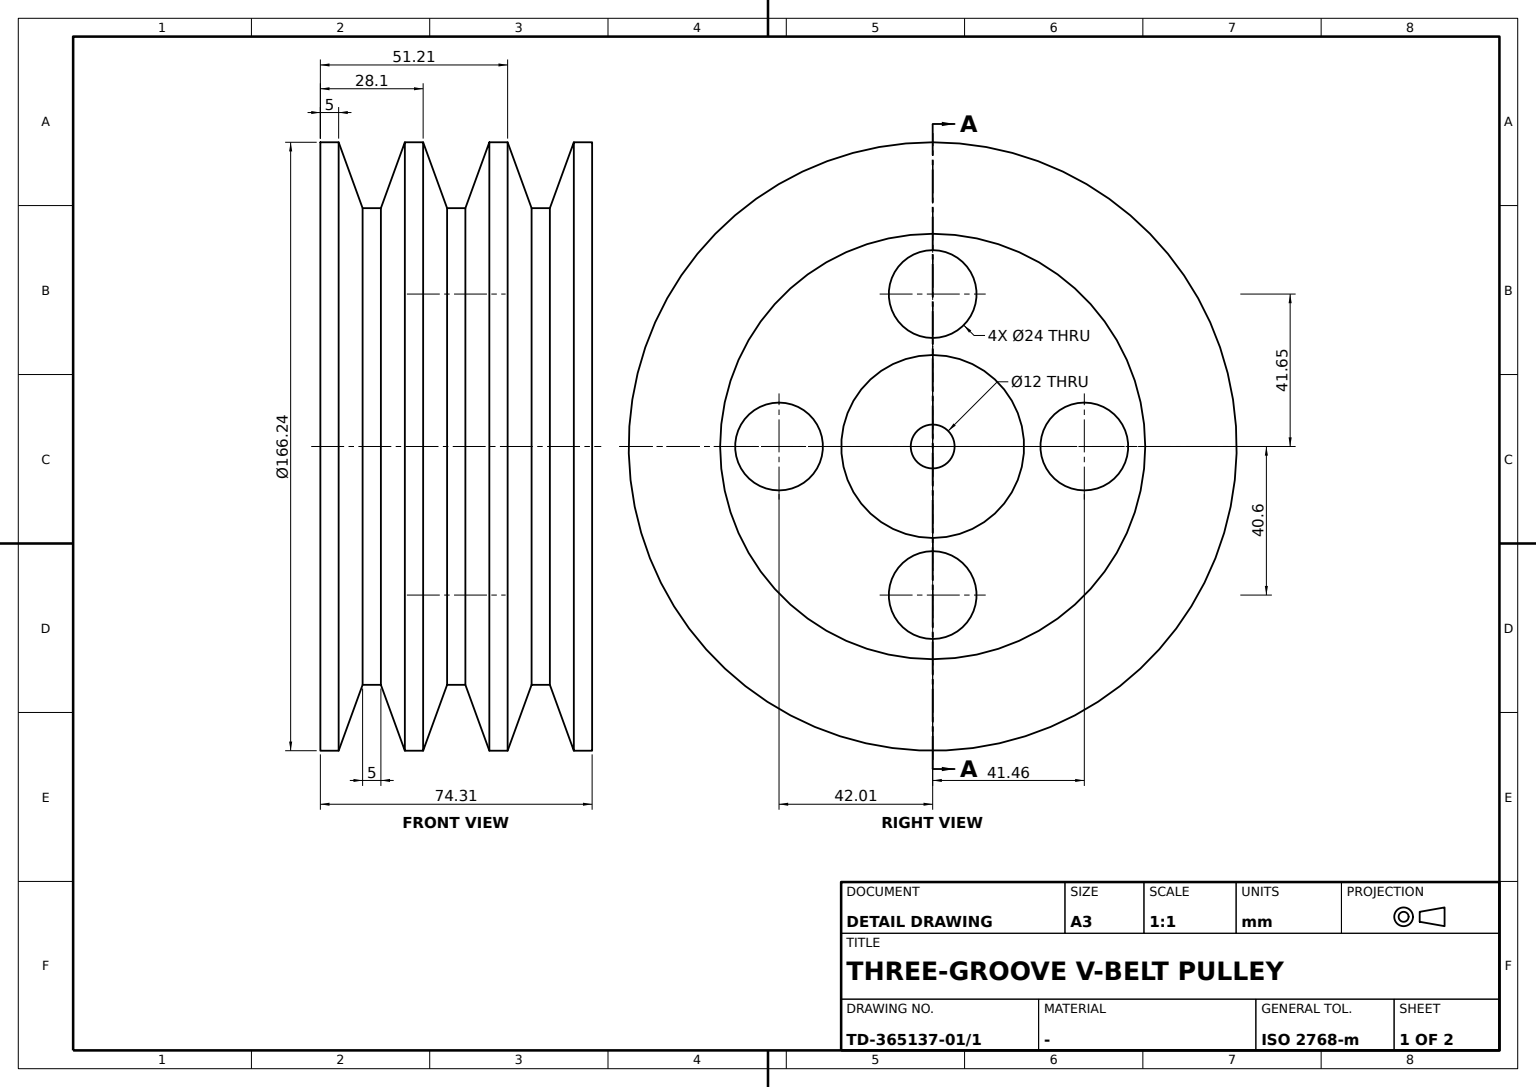
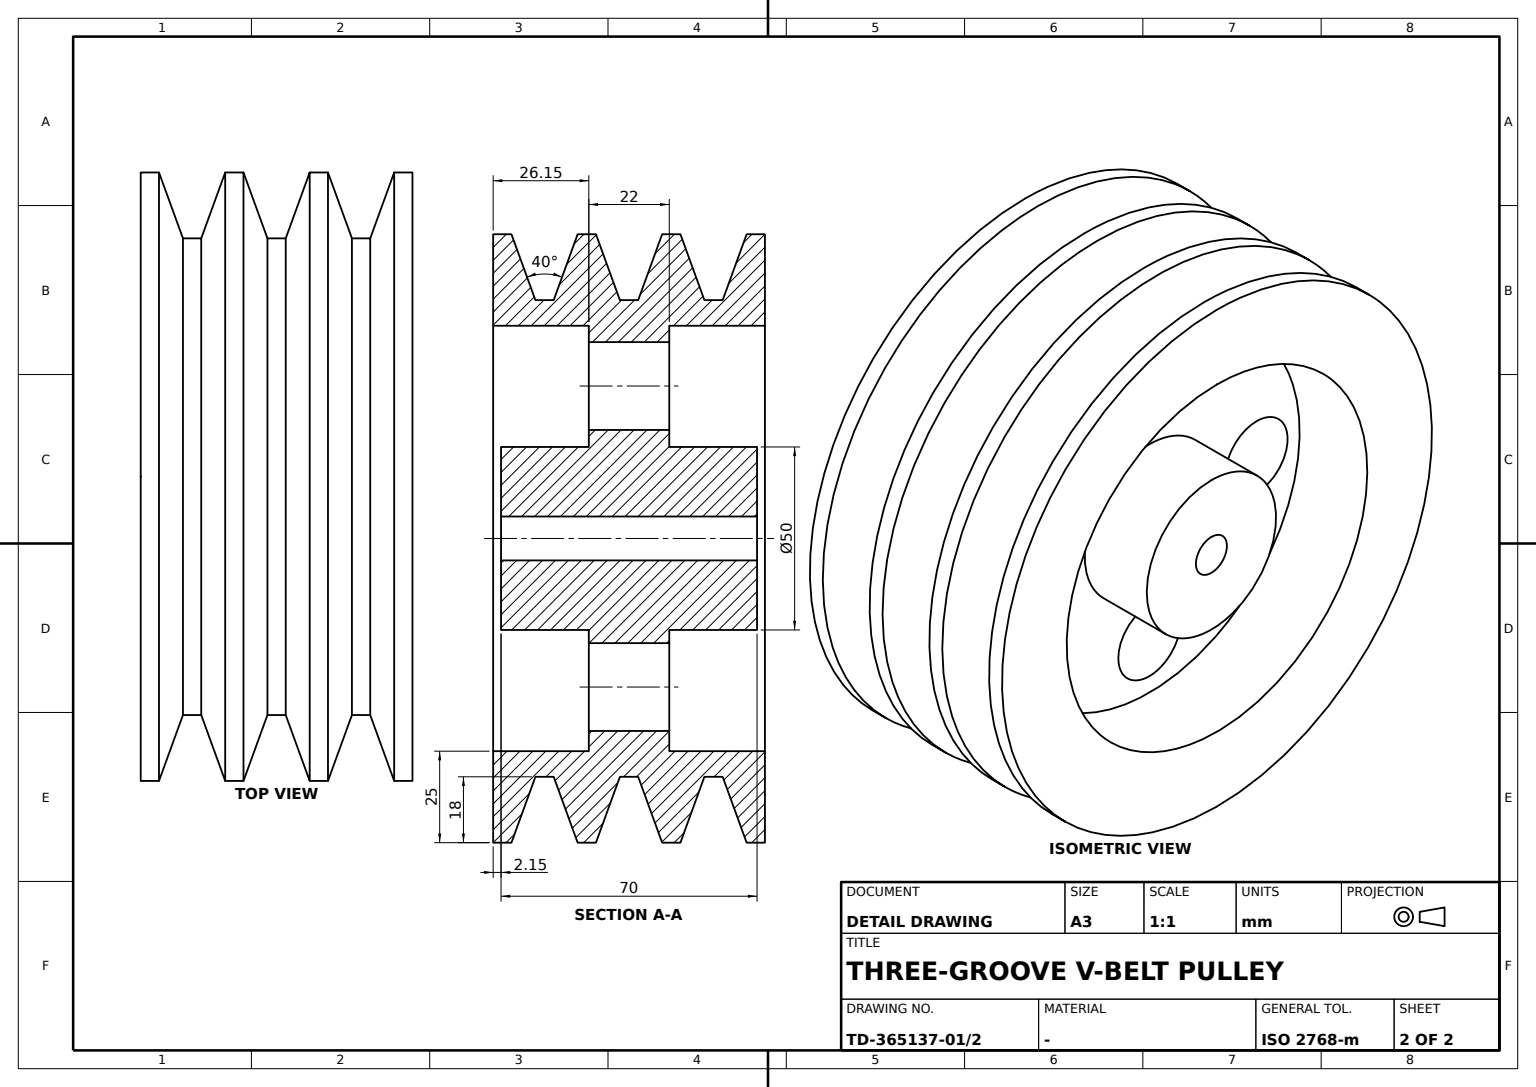
CATIA V5 part; units mm, degrees
sketch "Sketch1" plane through (0, 0, 0) normal (1, 0, 0) x (0, 1, 0)
  line L0 (0, 94.58) -> (0, -41.0411) construction
  point P0 (0, 94.58)
  point P1 (0, 65.1212)
  line L1 (0, 65.1212) -> (-2.5, 65.1212)
  point P2 (-2.5, 65.1212)
  line L2 (-2.5, 65.1212) -> (-9.0515, 83.1212)
  point P3 (-9.0515, 83.1212)
  line L3 (-9.0515, 83.1212) -> (-14.0515, 83.1212)
  point P4 (-14.0515, 83.1212)
  line L4 (-14.0515, 83.1212) -> (-20.6029, 65.1212)
  point P5 (-20.6029, 65.1212)
  line L5 (-20.6029, 65.1212) -> (-25.6029, 65.1212)
  point P6 (-25.6029, 65.1212)
  line L6 (-25.6029, 65.1212) -> (-32.1544, 83.1212)
  point P7 (-32.1544, 83.1212)
  line L7 (-32.1544, 83.1212) -> (-37.1544, 83.1212)
  point P8 (-37.1544, 83.1212)
  line L8 (-37.1544, 83.1212) -> (-37.1544, 58.1212)
  point P9 (-37.1544, 58.1212)
  line L9 (-37.1544, 58.1212) -> (-11, 58.1212)
  point P10 (-11, 58.1212)
  line L10 (-11, 58.1212) -> (-11, 25)
  point P11 (-11, 25)
  line L11 (-11, 25) -> (-35, 25)
  point P12 (-35, 25)
  line L12 (-35, 25) -> (-35, 6)
  point P13 (-35, 6)
  line L13 (-35, 6) -> (0, 6)
  point P14 (0, 6)
  point P15 (0, 94.58)
  point P16 (0, 65.1212)
  point P17 (2.5, 65.1212)
  point P18 (9.0515, 83.1212)
  point P19 (14.0515, 83.1212)
  point P20 (20.6029, 65.1212)
  point P21 (25.6029, 65.1212)
  point P22 (32.1544, 83.1212)
  point P23 (37.1544, 83.1212)
  point P24 (37.1544, 58.1212)
  point P25 (11, 58.1212)
  point P26 (11, 25)
  point P27 (35, 25)
  point P28 (35, 6)
  point P29 (0, 6)
  line L14 (0, 65.1212) -> (2.5, 65.1212)
  line L15 (2.5, 65.1212) -> (9.0515, 83.1212)
  line L16 (9.0515, 83.1212) -> (14.0515, 83.1212)
  line L17 (14.0515, 83.1212) -> (20.6029, 65.1212)
  line L18 (20.6029, 65.1212) -> (25.6029, 65.1212)
  line L19 (25.6029, 65.1212) -> (32.1544, 83.1212)
  line L20 (32.1544, 83.1212) -> (37.1544, 83.1212)
  line L21 (37.1544, 83.1212) -> (37.1544, 58.1212)
  line L22 (37.1544, 58.1212) -> (11, 58.1212)
  line L23 (11, 58.1212) -> (11, 25)
  line L24 (11, 25) -> (35, 25)
  line L25 (35, 25) -> (35, 6)
  line L26 (35, 6) -> (0, 6)
  dimension "length L1" = 2.5
  dimension "distance x axis L13" = 6
  dimension "distance L11 x axis" = 25
  dimension "distance L10 L0" = 11
  dimension "distance L0 L12" = 35
  dimension "angle L4 L2" = 40
  dimension "angle L2 L0" = 20
  dimension "length L7" = 5
  dimension "length L5" = 5
  dimension "distance L5 P8" = 18
  dimension "length L3" = 5
  dimension "distance L7 L9" = 25
  dimension "angle L6 L4" = 40
  constraint coincidence P0 y-axis
  constraint coincidence P1 L0
  constraint coincidence P5 L1
  constraint coincidence P7 L3
  constraint coincidence P11 L6
  constraint coincidence P14 L0
  constraint coincidence P1 P16
  constraint coincidence P14 P29
  constraint vertical L0 y-axis
  constraint vertical L8 y-axis
  constraint vertical L10 y-axis
  constraint vertical L12 y-axis
  constraint horizontal L1 x-axis
  constraint horizontal L3 x-axis
  constraint horizontal L5 x-axis
  constraint horizontal L7 x-axis
  constraint horizontal L9 x-axis
  constraint horizontal L11 x-axis
  constraint horizontal L13 x-axis
  constraint symmetry P0 P15 y-axis
  constraint symmetry P1 P16 y-axis
  constraint symmetry P2 P17 y-axis
  constraint symmetry P3 P18 y-axis
  constraint symmetry P4 P19 y-axis
  constraint symmetry P5 P20 y-axis
  constraint symmetry P6 P21 y-axis
  constraint symmetry P7 P22 y-axis
  constraint symmetry P8 P23 y-axis
  constraint symmetry P9 P24 y-axis
  constraint symmetry P10 P25 y-axis
  constraint symmetry P11 P26 y-axis
  constraint symmetry P12 P27 y-axis
  constraint symmetry P13 P28 y-axis
  constraint symmetry P14 P29 y-axis
  constraint symmetry L1 L14 y-axis
  constraint symmetry L2 L15 y-axis
  constraint symmetry L3 L16 y-axis
  constraint symmetry L4 L17 y-axis
  constraint symmetry L5 L18 y-axis
  constraint symmetry L6 L19 y-axis
  constraint symmetry L7 L20 y-axis
  constraint symmetry L8 L21 y-axis
  constraint symmetry L9 L22 y-axis
  constraint symmetry L10 L23 y-axis
  constraint symmetry L11 L24 y-axis
  constraint symmetry L12 L25 y-axis
  constraint symmetry L13 L26 y-axis
revolve "Shaft1" add sketch "Sketch1" angle 360 about axis through (0, 0, 0) along (0, 1, 0)
sketch "Sketch2" plane through (0, -35, 0) normal (0, -1, 0) x (1, 0, 0)
  circle A0 centre (42.0136, 0) radius 12
  point P0 (42.0136, 0)
  circle A1 centre (-41.4628, 0) radius 12
  point P1 (-41.4628, 0)
  circle A2 centre (0, 41.6485) radius 12
  point P2 (0, 41.6485)
  circle A3 centre (0, -40.5969) radius 12
  point P3 (0, -40.5969)
  dimension "radius A2" = 12
  dimension "radius A1" = 12
  dimension "radius A3" = 12
  dimension "radius A0" = 12
  constraint coincidence P0 x-axis
  constraint coincidence P1 x-axis
  constraint coincidence P2 y-axis
  constraint coincidence P3 y-axis
extrude "Pocket1" cut sketch "Sketch2" against normal through all
